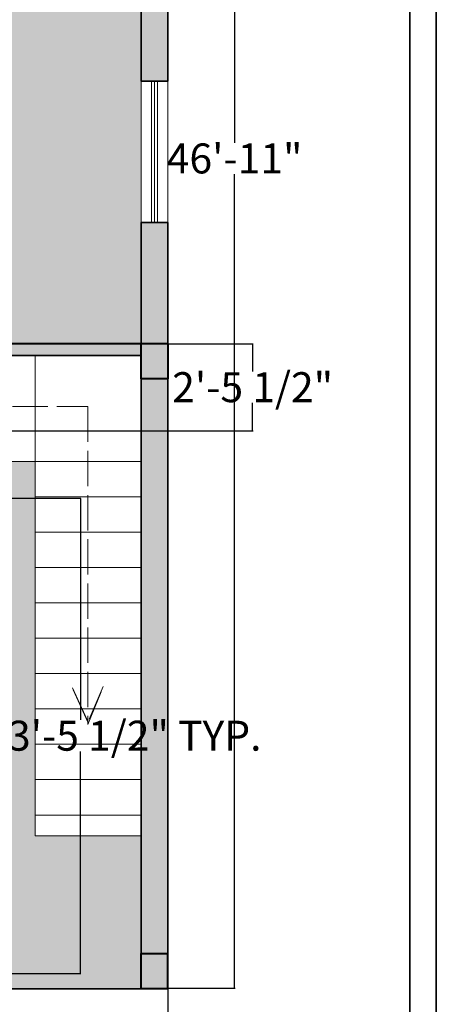
# Model space of a CAD drawing. Units: inches. Extents: x 1077 to 2505, y 1892 to 2728.
# Tile 24 of 26: x 2364 to 2505, y 2089 to 2423. Entities that reach past the tile are written whole.
import ezdxf

# ---------------------------------------------------------------- set-up
doc = ezdxf.new("R2010")
doc.units = ezdxf.units.IN
doc.linetypes.add('ACAD_ISO02W100', pattern=[15, 12, -3])
doc.layers.get('Defpoints').update_dxf_attribs({"color": 220, "linetype": 'ACAD_ISO02W100'})
for name, color, linetype, lineweight in [('A-ANNO-DIMS', 2, 'Continuous', 18), ('A-ANNO-STRS', 220, 'ACAD_ISO02W100', 13), ('A-ANNO-TTLB', 7, 'Continuous', 35), ('A-COLS', 7, 'Continuous', 40), ('A-FLOR-STRS', 7, 'Continuous', 18), ('A-WALL-PATT', 7, 'Continuous', 9), ('WALL', 7, 'Continuous', 35), ('WINDOW', 160, 'Continuous', 13)]:
    doc.layers.add(name, color=color, linetype=linetype, lineweight=lineweight)
doc.layers.add('A-FLOR-PATT', color=254, linetype='Continuous', lineweight=9, true_color=0xd7ebd2)
doc.styles.get("Standard").update_dxf_attribs({"font": 'arial.ttf'})
doc.dimstyles.get("Standard").update_dxf_attribs({"dimtxt": 10.18, "dimasz": 0.18, "dimexe": 0.18, "dimexo": 0.0625, "dimgap": 0.09, "dimtad": 0, "dimtih": 1, "dimtoh": 1, "dimdec": 0, "dimzin": 0, "dimdsep": 46, "dimlunit": 3, "dimtxsty": 'Standard', "dimcen": 0.09, "dimadec": 0, "dimazin": 0, "dimtfac": 1, "dimtdec": 0, "dimtofl": 0, "dimtmove": 0, "dimatfit": 3, "dimfxl": 1, "dimtolj": 1, "dimtzin": 0, "dimarcsym": 0})

# ---------------------------------------------------------------- blocks, each defined once
blk = doc.blocks.new('C1')
h = blk.add_hatch(color=256)
h.dxf.hatch_style = 1
h.paths.add_polyline_path([(1668.56, 2445.41), (1677.56, 2445.41), (1677.56, 2457.41), (1668.56, 2457.41)])
for p, q in [((1668.56, 2457.41), (1677.56, 2457.41)), ((1668.56, 2445.41), (1668.56, 2457.41)), ((1677.56, 2457.41), (1677.56, 2445.41)), ((1677.56, 2445.41), (1668.56, 2445.41))]:
    blk.add_line(p, q)
blk = doc.blocks.new('*D19')
at = {"layer": 'A-ANNO-DIMS', "color": 0, "lineweight": -2, "transparency": 16777216}
for p, q in [((2412.91, 2657.64), (2436.75, 2657.64)), ((2436.57, 2657.46), (2436.57, 2381.28)), ((2436.57, 2094.52), (2436.57, 2370.7)), ((2412.91, 2094.34), (2436.75, 2094.34))]:
    blk.add_line(p, q, dxfattribs=at)
at = {"layer": 'A-ANNO-DIMS', "color": 0, "transparency": 16777216}
for points in [[(2436.54, 2657.46), (2436.6, 2657.46), (2436.57, 2657.64)], [(2436.54, 2094.52), (2436.6, 2094.52), (2436.57, 2094.34)]]:
    blk.add_solid(points, dxfattribs=at)
at = {"layer": 'Defpoints', "color": 0, "transparency": 16777216}
for p in [(2412.85, 2657.64), (2412.85, 2094.34), (2436.57, 2094.34)]:
    blk.add_point(p, dxfattribs=at)
at = {"layer": 'A-ANNO-DIMS', "color": 0, "transparency": 16777216, "insert": (2436.57, 2375.99), "char_height": 10.18, "attachment_point": 5}
blk.add_mtext('\\A1;46\'-11"', dxfattribs=at)
blk = doc.blocks.new('WINDOW-48-EXT')
for p, q in [((0, 48), (0, 0)), ((3.5, 48), (3.5, 0)), ((4.5, 48), (4.5, 0)), ((5.5, 48), (5.5, 0)), ((9, 0), (9, 48))]:
    blk.add_line(p, q)
blk = doc.blocks.new('STAIR-PLAN-RETURN')
for p, q in [((0, 163.08), (0, 127.08)), ((12, 163.08), (12, 127.08)), ((24, 163.08), (24, 127.08)), ((36, 163.08), (36, 0)), ((36, 163.08), (36, 127.08)), ((0, 127.08), (72, 127.08)), ((36, 115.08), (72, 115.08)), ((36, 103.08), (72, 103.08)), ((36, 91.08), (72, 91.08)), ((36, 79.08), (72, 79.08)), ((36, 67.08), (72, 67.08)), ((36, 55.08), (72, 55.08)), ((36, 43.08), (72, 43.08)), ((36, 31.08), (72, 31.08)), ((36, 19.08), (72, 19.08)), ((36, 7.08), (72, 7.08)), ((72, 0), (36, 0))]:
    blk.add_line(p, q)
blk = doc.blocks.new('STAIR-DIRECTION')
for p, q in [((0, 107.9), (70.51, 107.9)), ((70.51, 107.9), (70.51, 0)), ((70.51, 0.8), (65.28, 12.48)), ((65.28, 12.48), (70.51, 1.21)), ((70.51, 0), (75.75, 12.88)), ((75.75, 12.88), (70.51, 0.8))]:
    blk.add_line(p, q)
blk = doc.blocks.new('SHEET-FRAME-RESIDENTIAL')
for points in [[(0, 830.04), (543.52, 830.04), (543.52, 0), (0, 0)], [(9, 821.04), (534.52, 821.04), (534.52, 9), (9, 9)]]:
    blk.add_lwpolyline(points, close=True)
blk = doc.blocks.new('*D56')
at = {"layer": 'A-ANNO-DIMS', "color": 0, "lineweight": -2, "transparency": 16777216}
for p, q in [((2360.05, 2260.72), (2384.37, 2260.72)), ((2384.19, 2260.54), (2384.19, 2185.41)), ((2384.19, 2099.57), (2384.19, 2174.7)), ((2360.05, 2099.39), (2384.37, 2099.39))]:
    blk.add_line(p, q, dxfattribs=at)
at = {"layer": 'A-ANNO-DIMS', "color": 0, "transparency": 16777216}
for points in [[(2384.16, 2260.54), (2384.22, 2260.54), (2384.19, 2260.72)], [(2384.16, 2099.57), (2384.22, 2099.57), (2384.19, 2099.39)]]:
    blk.add_solid(points, dxfattribs=at)
at = {"layer": 'Defpoints', "color": 0, "transparency": 16777216}
for p in [(2359.99, 2260.72), (2384.19, 2260.72), (2359.99, 2099.39)]:
    blk.add_point(p, dxfattribs=at)
at = {"layer": 'A-ANNO-DIMS', "color": 0, "transparency": 16777216, "insert": (2384.19, 2180.06), "char_height": 10.18, "attachment_point": 5}
blk.add_mtext('\\A1;CAR 13\'-5 1/2" TYP.', dxfattribs=at)
blk = doc.blocks.new('*D57')
at = {"layer": 'A-ANNO-DIMS', "color": 0, "lineweight": -2, "transparency": 16777216}
for p, q in [((2293.39, 2099.33), (2293.39, 2075.01)), ((2359.99, 2099.33), (2359.99, 2075.01)), ((2293.57, 2075.19), (2359.81, 2075.19)), ((2359.99, 2075.19), (2360.17, 2075.19))]:
    blk.add_line(p, q, dxfattribs=at)
at = {"layer": 'A-ANNO-DIMS', "color": 0, "transparency": 16777216}
for points in [[(2293.57, 2075.22), (2293.57, 2075.16), (2293.39, 2075.19)], [(2359.81, 2075.22), (2359.81, 2075.16), (2359.99, 2075.19)]]:
    blk.add_solid(points, dxfattribs=at)
at = {"layer": 'Defpoints', "color": 0, "transparency": 16777216}
for p in [(2293.39, 2099.39), (2359.99, 2099.39), (2359.99, 2075.19)]:
    blk.add_point(p, dxfattribs=at)
at = {"layer": 'A-ANNO-DIMS', "color": 0, "transparency": 16777216, "insert": (2403.15, 2075.19), "char_height": 10.18, "attachment_point": 5}
blk.add_mtext('\\A1;5\'-6 1/2" TYP.', dxfattribs=at)
blk = doc.blocks.new('*D63')
at = {"layer": 'A-ANNO-DIMS', "color": 0, "lineweight": -2, "transparency": 16777216}
for p, q in [((2035.85, 2094.07), (2035.85, 2065.11)), ((2413.85, 2094.07), (2413.85, 2065.11)), ((2036.03, 2065.29), (2207.27, 2065.29)), ((2413.67, 2065.29), (2242.42, 2065.29))]:
    blk.add_line(p, q, dxfattribs=at)
at = {"layer": 'A-ANNO-DIMS', "color": 0, "transparency": 16777216}
for points in [[(2036.03, 2065.32), (2036.03, 2065.26), (2035.85, 2065.29)], [(2413.67, 2065.32), (2413.67, 2065.26), (2413.85, 2065.29)]]:
    blk.add_solid(points, dxfattribs=at)
at = {"layer": 'Defpoints', "color": 0, "transparency": 16777216}
for p in [(2035.85, 2094.14), (2413.85, 2094.14), (2413.85, 2065.29)]:
    blk.add_point(p, dxfattribs=at)
at = {"layer": 'A-ANNO-DIMS', "color": 0, "transparency": 16777216, "insert": (2224.85, 2065.29), "char_height": 10.18, "attachment_point": 5}
blk.add_mtext('\\A1;31\'-6"', dxfattribs=at)
blk = doc.blocks.new('*D72')
at = {"layer": 'A-ANNO-DIMS', "color": 0, "lineweight": -2, "transparency": 16777216}
for p, q in [((2280.86, 2313.12), (2442.88, 2313.12)), ((2442.7, 2312.94), (2442.7, 2303.7)), ((2442.7, 2283.76), (2442.7, 2292.99)), ((2285.24, 2283.58), (2442.88, 2283.58))]:
    blk.add_line(p, q, dxfattribs=at)
at = {"layer": 'A-ANNO-DIMS', "color": 0, "transparency": 16777216}
for points in [[(2442.67, 2312.94), (2442.73, 2312.94), (2442.7, 2313.12)], [(2442.67, 2283.76), (2442.73, 2283.76), (2442.7, 2283.58)]]:
    blk.add_solid(points, dxfattribs=at)
at = {"layer": 'Defpoints', "color": 0, "transparency": 16777216}
for p in [(2280.8, 2313.12), (2285.18, 2283.58), (2442.7, 2283.58)]:
    blk.add_point(p, dxfattribs=at)
at = {"layer": 'A-ANNO-DIMS', "color": 0, "transparency": 16777216, "insert": (2442.7, 2298.35), "char_height": 10.18, "attachment_point": 5}
blk.add_mtext('\\A1;2\'-5 1/2"', dxfattribs=at)

msp = doc.modelspace()

# ---------------------------------------------------------------- hatches: boundary and pattern name
at = {"layer": 'A-FLOR-PATT', "transparency": 33554559}
h = msp.add_hatch(color=256, dxfattribs=at)
h.dxf.hatch_style = 1
h.paths.add_polyline_path([(2252.85, 2583.14), (2232.15, 2583.14), (2208.15, 2583.17), (2208.15, 2583.14), (2186.85, 2583.14), (2186.85, 2486.14), (2186.85, 2475.14), (2182.85, 2475.14), (2182.85, 2521.11), (2164.84, 2521.11), (2164.84, 2583.14), (2126.63, 2583.14), (2078.63, 2583.13), (2078.63, 2583.14), (2044.85, 2583.14), (2044.85, 2439.14), (2146.85, 2439.14), (2146.85, 2435.14), (2120.85, 2435.14), (2044.85, 2435.14), (2044.85, 2401), (2044.85, 2401), (2044.85, 2377), (2044.85, 2377), (2044.85, 2313.14), (2116.85, 2313.14), (2116.85, 2405.14), (2120.85, 2405.14), (2120.85, 2313.14), (2146.85, 2313.14), (2146.85, 2312.21), (2182.85, 2312.21), (2182.85, 2313.14), (2186.85, 2313.14), (2186.85, 2312.21), (2222.85, 2312.21), (2222.85, 2313.14), (2289.85, 2313.14), (2289.85, 2094.14), (2404.85, 2094.14), (2404.85, 2146.06), (2368.85, 2146.06), (2368.85, 2273.14), (2332.85, 2273.14), (2332.85, 2309.14), (2325.85, 2309.14), (2325.85, 2313.14), (2404.85, 2313.14), (2404.85, 2354.2), (2404.85, 2402.2), (2404.85, 2435.14), (2292.85, 2435.14), (2292.85, 2439.14), (2333.66, 2439.14), (2333.66, 2457.16), (2404.85, 2457.16), (2404.85, 2583.14), (2356.85, 2583.14), (2356.85, 2592.14), (2404.85, 2592.14), (2404.85, 2648.14), (2375.5, 2648.14), (2375.5, 2648.03), (2351.47, 2648.03), (2351.47, 2648.14), (2326.85, 2648.14), (2326.85, 2583.14), (2256.85, 2583.14), (2256.85, 2435.14), (2182.85, 2435.14), (2182.85, 2439.14), (2186.85, 2439.14), (2252.85, 2439.14), (2252.85, 2486.14), (2216.85, 2486.14), (2216.85, 2490.14), (2252.85, 2490.14)])
h.paths.add_polyline_path([(2214.97, 2488.05), (2212.97, 2488.05), (2212.97, 2487.05, 0.414214), (2213.97, 2486.05), (2201.97, 2486.05), (2201.97, 2483.04), (2200.58, 2483.04), (2200.58, 2486.05), (2187.97, 2486.05, -0.414214), (2186.97, 2487.05), (2186.97, 2490.05), (2188.97, 2490.05), (2188.97, 2516.05, -0.446908)], flags=16)
h.paths.add_polyline_path([(2162.4, 2565.16), (2146.2, 2565.16), (2146.2, 2581.36), (2162.4, 2581.36)], flags=16)
h.paths.add_polyline_path([(2161.5, 2566.06), (2147.1, 2566.06), (2147.1, 2580.46), (2161.5, 2580.46)], flags=0)
h.paths.add_polyline_path([(2145.3, 2506.66, -0.414214), (2144.4, 2505.76), (2122.45, 2505.76), (2081.4, 2505.76, -0.414214), (2080.5, 2506.66), (2080.5, 2563.14), (2080.5, 2577.72), (2080.5, 2581.36), (2145.3, 2581.36), (2145.3, 2577.72), (2144.4, 2577.72, -0.414214), (2145.3, 2576.82)], flags=16)
h.paths.add_polyline_path([(2150.3, 2575.03, -1), (2158.24, 2575.03, -1)], flags=0)
h.paths.add_polyline_path([(2150.64, 2575.03, -1), (2157.89, 2575.03, -1)], flags=0)
h.paths.add_polyline_path([(2180.11, 2468.19), (2180.11, 2437.69), (2180.36, 2436.69), (2180.36, 2437.69), (2179.11, 2437.69), (2179.11, 2468.17, 0.404641), (2149.61, 2437.69), (2149.36, 2436.69, -0.414214), (2148.86, 2436.19), (2148.36, 2436.19), (2148.36, 2435.69, -0.414214), (2147.86, 2435.19), (2146.86, 2435.19), (2146.86, 2440.19), (2147.86, 2440.19, -0.414214), (2148.36, 2439.69), (2148.36, 2439.19), (2148.86, 2439.19, -0.414214), (2149.36, 2438.69), (2149.61, 2437.69, -0.414214)], flags=16)
h.paths.add_polyline_path([(2145.14, 2554.26, 0.292232), (2136.49, 2542.78, 0.052719), (2081.25, 2554.26), (2080.6, 2554.26), (2080.6, 2563.14), (2081.25, 2563.14), (2102.73, 2563.14, -0.117785), (2103.09, 2563.91, -0.059418), (2112.19, 2573, -0.379859), (2114.6, 2572.86, -0.02509), (2118.73, 2569.3, -0.025935), (2122.97, 2573, -0.379859), (2125.38, 2572.86, -0.061767), (2134.84, 2563.41, -0.069393), (2135.14, 2563.14), (2145.14, 2563.14)], flags=0)
h.paths.add_polyline_path([(2120.79, 2554.26), (2117.88, 2554.26, -0.015371), (2115.33, 2552.11, -0.429576), (2112.69, 2552.04, -0.016036), (2110.01, 2554.26), (2080.6, 2554.26), (2080.6, 2560.4), (2104.1, 2560.4, 0.055344), (2112.69, 2552.04, 0.331768), (2114.84, 2551.72, 0.027343), (2119.32, 2555.62, 0.00919)], flags=0)
h.paths.add_polyline_path([(2152.88, 2574.32), (2154.19, 2575.07), (2154.19, 2576.58, 0.399698), (2152.71, 2575.03, 0.119004)], flags=0)
h.paths.add_polyline_path([(2152.53, 2575.03, -1), (2156, 2575.03, -1)], flags=0)
h.paths.add_polyline_path([(2154.27, 2574.94), (2154.34, 2574.98), (2154.34, 2575.07), (2154.3, 2575.09), (2154.23, 2574.96)], flags=0)
h.paths.add_polyline_path([(2259.6, 2468.17, -0.414214), (2290.1, 2437.67), (2290.35, 2438.67), (2290.1, 2437.67, 0.404641), (2260.6, 2468.15), (2260.6, 2437.67), (2259.35, 2437.67), (2259.35, 2436.67, -0.414214), (2258.85, 2436.17), (2258.35, 2436.17), (2258.35, 2435.67, -0.414214), (2257.85, 2435.17), (2256.85, 2435.17), (2256.85, 2440.17), (2257.85, 2440.17, -0.414214), (2258.35, 2439.67), (2258.35, 2439.17), (2258.85, 2439.17, -0.414214), (2259.35, 2438.67)], flags=16)
h.paths.add_polyline_path([(2327.48, 2541.19, -0.414214), (2328.38, 2542.09), (2384.85, 2542.09), (2399.43, 2542.09), (2403.08, 2542.09), (2403.08, 2477.29), (2399.43, 2477.29), (2399.43, 2478.19, -0.414214), (2398.53, 2477.29), (2328.38, 2477.29, -0.414214), (2327.48, 2478.19), (2327.48, 2500.14)], flags=16)
h.paths.add_polyline_path([(2340.38, 2542.09, 0.253465), (2337.43, 2532.13, 0.2538), (2327.47, 2529.17)], flags=16)
h.paths.add_polyline_path([(2080.5, 2518.67, 0.253465), (2090.46, 2515.72, 0.2538), (2093.42, 2505.75)], flags=16)
h.paths.add_polyline_path([(2327.09, 2584.7), (2327.09, 2587.7), (2329.09, 2587.7), (2329.09, 2613.7, -0.01951), (2331.09, 2613.66), (2331.09, 2585.7), (2331.09, 2584.7, -0.414214), (2330.09, 2583.7), (2328.09, 2583.7, -0.414214)], flags=16)
h.paths.add_polyline_path([(2239.78, 2404.11), (2252.36, 2404.11), (2252.36, 2405.72), (2239.78, 2405.72)], flags=16)
h.paths.add_polyline_path([(2237.26, 2403.16), (2237.26, 2395.8), (2237.82, 2395.8), (2237.82, 2402.03, -0.41429), (2238.38, 2402.59), (2253.79, 2402.59, -0.414213), (2254.35, 2402.03), (2254.35, 2395.8), (2254.91, 2395.8), (2254.91, 2403.16)], flags=16)
h.paths.add_polyline_path([(2120.69, 2434.12), (2120.69, 2432.12, -0.414214), (2119.69, 2431.12), (2118.69, 2431.12), (2090.73, 2431.12, 0.400854), (2116.69, 2407.02), (2116.69, 2407.12), (2118.69, 2407.12, -0.446908), (2090.69, 2433.12), (2116.69, 2433.12), (2116.69, 2435.12), (2119.69, 2435.12, -0.414214)], flags=16)
h.paths.add_polyline_path([(2262.11, 2404.11), (2274.69, 2404.11), (2274.69, 2405.72), (2262.11, 2405.72)], flags=16)
h.paths.add_polyline_path([(2259.59, 2403.16), (2262.11, 2404.11), (2274.69, 2404.11), (2277.24, 2403.16)], flags=16)
h.paths.add_polyline_path([(2289.58, 2389.14), (2289.58, 2376.57), (2291.19, 2376.57), (2291.19, 2389.14)], flags=16)
h.paths.add_polyline_path([(2288.62, 2391.67), (2281.15, 2391.67), (2281.15, 2391.11), (2287.5, 2391.11, -0.41429), (2288.06, 2390.54), (2288.06, 2375.14, -0.414237), (2287.5, 2374.58), (2281.15, 2374.58), (2281.15, 2374.01), (2288.62, 2374.01)], flags=16)
h.paths.add_polyline_path([(2274.69, 2357.14), (2274.69, 2355.52), (2276.22, 2355.52, 0.414236), (2277.24, 2356.54), (2277.24, 2358.09)], flags=16)
h.paths.add_polyline_path([(2252.36, 2357.14), (2252.36, 2355.52), (2253.89, 2355.52, 0.414235), (2254.91, 2356.54), (2254.91, 2358.09)], flags=16)
h.paths.add_polyline_path([(2224.02, 2376.03), (2222.41, 2376.03), (2222.41, 2374.5, 0.414235), (2223.43, 2373.48), (2224.98, 2373.48)], flags=16)
h.paths.add_polyline_path([(2276.68, 2365.45), (2276.68, 2359.22, -0.41419), (2276.12, 2358.66), (2260.71, 2358.66, -0.414137), (2260.15, 2359.22), (2260.15, 2365.45), (2254.35, 2365.45), (2254.35, 2359.22, -0.414189), (2253.79, 2358.66), (2238.38, 2358.66, -0.414137), (2237.82, 2359.22), (2237.82, 2365.45)], flags=16)
h.paths.add_polyline_path([(2079.6, 2565.16), (2063.4, 2565.16), (2063.4, 2581.36), (2079.6, 2581.36)], flags=16)
h.paths.add_polyline_path([(2078.7, 2566.06), (2064.3, 2566.06), (2064.3, 2580.46), (2078.7, 2580.46)], flags=0)
h.paths.add_polyline_path([(2339.31, 2583.7), (2339.31, 2586.71), (2340.7, 2586.71), (2340.7, 2583.7), (2342.09, 2583.7), (2342.09, 2580.7), (2340.7, 2580.7), (2340.7, 2583.7)], flags=16)
h.paths.add_polyline_path([(2123.69, 2421.51), (2123.69, 2420.12), (2120.69, 2420.12), (2120.69, 2421.51), (2117.68, 2421.51), (2117.68, 2422.89), (2120.69, 2422.89), (2120.69, 2421.51)], flags=16)
h.paths.add_polyline_path([(2067.57, 2575.03, -1), (2075.51, 2575.03, -1)], flags=0)
h.paths.add_polyline_path([(2067.92, 2575.03, -1), (2075.17, 2575.03, -1)], flags=0)
h.paths.add_polyline_path([(2070.16, 2574.32), (2071.47, 2575.07), (2071.47, 2576.58, 0.399698), (2069.99, 2575.03, 0.119004)], flags=0)
h.paths.add_polyline_path([(2069.81, 2575.03, -1), (2073.28, 2575.03, -1)], flags=0)
h.paths.add_polyline_path([(2071.54, 2574.94), (2071.62, 2574.89), (2071.62, 2574.98)], flags=0)
h.paths.add_polyline_path([(2364.5, 2486.1, 0.052719), (2375.98, 2541.34), (2375.98, 2541.99), (2384.85, 2541.99), (2384.85, 2541.34), (2384.85, 2519.86, -0.117785), (2385.62, 2519.51, -0.059418), (2394.72, 2510.41, -0.379859), (2394.58, 2507.99, -0.02509), (2391.01, 2503.87, -0.025935), (2394.72, 2499.62, -0.379859), (2394.58, 2497.21, -0.061767), (2385.12, 2487.75, -0.069393), (2384.85, 2487.45), (2384.85, 2477.45), (2375.98, 2477.45, 0.292232)], flags=0)
h.paths.add_polyline_path([(2373.75, 2509.9, -0.016036), (2375.98, 2512.58), (2375.98, 2541.99), (2382.12, 2541.99), (2382.12, 2518.49, 0.055344), (2373.75, 2509.9, 0.331768), (2373.44, 2507.75, 0.027343), (2377.33, 2503.27, 0.00919), (2375.98, 2501.8), (2375.98, 2504.71, -0.015371), (2373.82, 2507.26, -0.429576)], flags=0)
h.paths.add_polyline_path([(2356.95, 2631.48, -0.171636), (2360.13, 2636.99), (2360.13, 2639.35), (2356, 2639.35, -0.414214), (2355.01, 2640.34), (2355.01, 2646.64, -0.414214), (2356, 2647.62), (2372.14, 2647.62, -0.414214), (2373.13, 2646.64), (2373.13, 2640.34, -0.414214), (2372.14, 2639.35), (2368.01, 2639.35), (2368.01, 2636.99, -0.171636), (2371.2, 2631.48, -0.258205), (2366.63, 2620.45), (2361.51, 2620.45, -0.258205)], flags=16)
h.paths.add_polyline_path([(2358.52, 2631.48, -0.171636), (2361.71, 2636.99), (2366.43, 2636.99, -0.171636), (2369.62, 2631.48, -0.210384), (2366.67, 2622), (2361.47, 2622, -0.210384)], flags=0)
h.paths.add_polyline_path([(2386.88, 2542.99), (2386.88, 2559.19), (2403.08, 2559.19), (2403.08, 2542.99)], flags=16)
h.paths.add_polyline_path([(2387.78, 2543.89), (2387.78, 2558.29), (2402.18, 2558.29), (2402.18, 2543.89)], flags=0)
h.paths.add_polyline_path([(2392.77, 2551.05, -1), (2400.71, 2551.05, -1)], flags=0)
h.paths.add_polyline_path([(2393.11, 2551.05, -1), (2400.37, 2551.05, -1)], flags=0)
h.paths.add_polyline_path([(2386.88, 2476.39), (2403.08, 2476.39), (2403.08, 2460.19), (2386.88, 2460.19)], flags=16)
h.paths.add_polyline_path([(2398.48, 2550.97), (2398.3, 2550.97, -0.544606), (2396.03, 2549.66), (2395.94, 2549.51, 0.547962)], flags=0)
h.paths.add_polyline_path([(2387.78, 2475.49), (2402.18, 2475.49), (2402.18, 2461.09), (2387.78, 2461.09)], flags=0)
h.paths.add_polyline_path([(2396.79, 2551.12), (2396.74, 2551.2), (2396.7, 2551.12)], flags=0)
h.paths.add_polyline_path([(2400.71, 2468.32, -1), (2392.77, 2468.32, -1)], flags=0)
h.paths.add_polyline_path([(2400.37, 2468.32, -1), (2393.11, 2468.32, -1)], flags=0)
h.paths.add_polyline_path([(2398.48, 2468.25), (2398.3, 2468.25, -0.544606), (2396.03, 2466.94), (2395.94, 2466.78, 0.547962)], flags=0)
h.paths.add_polyline_path([(2396.79, 2468.4), (2396.74, 2468.48), (2396.7, 2468.4)], flags=0)
h.paths.add_polyline_path([(2292.64, 2341.23, -0.414214), (2323.14, 2310.73), (2323.39, 2311.73), (2323.14, 2310.73, 0.404641), (2293.64, 2341.21), (2293.64, 2310.73), (2292.39, 2310.73), (2292.39, 2309.73, -0.414214), (2291.89, 2309.23), (2291.39, 2309.23), (2291.39, 2308.73, -0.414214), (2290.89, 2308.23), (2289.89, 2308.23), (2289.89, 2313.23), (2290.89, 2313.23, -0.414214), (2291.39, 2312.73), (2291.39, 2312.23), (2291.89, 2312.23, -0.414214), (2292.39, 2311.73)], flags=16)
h.paths.add_polyline_path([(2389.45, 2641.69), (2392.75, 2641.69), (2392.75, 2641.87), (2389.45, 2641.87)], flags=16)
edge = h.paths.add_edge_path(flags=16)
edge.add_arc((2393.3, 2638.65), 0.183, 270, 360)
edge.add_line((2393.49, 2638.65), (2393.49, 2645.8))
edge.add_line((2393.49, 2645.8), (2395.61, 2645.8))
edge.add_line((2395.61, 2645.8), (2395.61, 2647.8))
edge.add_line((2395.61, 2647.8), (2390.57, 2647.8))
edge.add_line((2390.57, 2647.8), (2390.57, 2645.8))
edge.add_line((2390.57, 2645.8), (2392.19, 2645.8))
edge.add_line((2392.19, 2645.8), (2392.19, 2644.98))
edge.add_line((2392.19, 2644.98), (2391.02, 2644.98))
edge.add_line((2391.02, 2644.98), (2391.02, 2645.8))
edge.add_line((2391.02, 2645.8), (2390.57, 2645.8))
edge.add_line((2390.57, 2645.8), (2390.57, 2647.8))
edge.add_line((2390.57, 2647.8), (2395.61, 2647.8))
edge.add_line((2395.61, 2647.8), (2395.61, 2647.32))
edge.add_line((2395.61, 2647.32), (2397.95, 2647.56))
edge.add_line((2397.95, 2647.56), (2397.95, 2647.8))
edge.add_line((2397.95, 2647.8), (2398.81, 2647.8))
edge.add_line((2398.81, 2647.8), (2398.81, 2647.23))
edge.add_line((2398.81, 2647.23), (2398.63, 2645.77))
edge.add_ellipse((2398.41, 2644.93), major_axis=(-1.08, 0), ratio=0.790849, start_angle=180, end_angle=255.2976, ccw=False)
edge.add_line((2399.49, 2644.93), (2399.49, 2644.36))
edge.add_ellipse((2398.41, 2644.36), major_axis=(-1.08, 0), ratio=0.790849, start_angle=0, end_angle=180, ccw=False)
edge.add_line((2397.32, 2644.36), (2397.33, 2644.85))
edge.add_ellipse((2398.41, 2644.93), major_axis=(-1.08, 0), ratio=0.790849, start_angle=284.7024, end_angle=364.0401, ccw=False)
edge.add_line((2398.1, 2645.73), (2398.1, 2647.23))
edge.add_line((2398.1, 2647.23), (2397.95, 2647.23))
edge.add_line((2397.95, 2647.23), (2395.61, 2646.99))
edge.add_line((2395.61, 2646.99), (2395.61, 2645.8))
edge.add_line((2395.61, 2645.8), (2393.49, 2645.8))
edge.add_line((2393.49, 2645.8), (2393.49, 2638.46))
edge.add_line((2393.49, 2638.46), (2393.3, 2638.46))
h.paths.add_polyline_path([(2353.64, 2256.32, -0.292371), (2356.22, 2253.81, -0.085148), (2358.52, 2214.83, -0.01331), (2357.59, 2104.48, -0.379287), (2354.54, 2101.26, -0.0502), (2298.86, 2101.26, -0.379287), (2295.81, 2104.48, -0.01331), (2294.88, 2214.83, -0.086132), (2297.28, 2254.24, -0.295116), (2299.9, 2256.76, -0.114238)], flags=16)
h.paths.add_polyline_path([(2352.48, 2211.82, -0.355389), (2354.02, 2208.08), (2350.26, 2195.63, -0.398275), (2346.44, 2193.45, 0.113332), (2306.96, 2193.45, -0.398275), (2303.14, 2195.63), (2299.38, 2208.08, -0.355394), (2300.92, 2211.82, -0.265725)], flags=0)
h.paths.add_polyline_path([(2297.68, 2201.7), (2303.26, 2187.65), (2303.26, 2166.61), (2298.16, 2163.24)], flags=0)
h.paths.add_polyline_path([(2355.78, 2201.7), (2355.31, 2163.24), (2350.2, 2166.61), (2350.2, 2187.65)], flags=0)
h.paths.add_polyline_path([(2303.26, 2164.35), (2303.26, 2143.1), (2298.44, 2128.54), (2298.19, 2161.01)], flags=0)
h.paths.add_polyline_path([(2350.2, 2164.35), (2355.28, 2161.01), (2355.03, 2128.54), (2350.2, 2143.1)], flags=0)
h.paths.add_polyline_path([(2347.2, 2136.38), (2351.71, 2113.65, -0.090102), (2301.76, 2113.63), (2306.27, 2136.37, 0.036636)], flags=0)
h.paths.add_polyline_path([(2304.86, 2165.32), (2354.76, 2165.32), (2354.76, 2183.87), (2304.86, 2183.87)], flags=8)
h.paths.add_polyline_path([(2053.76, 2360.82), (2103.97, 2360.82), (2103.97, 2394.41), (2053.76, 2394.41)], flags=24)
h.paths.add_polyline_path([(2153.41, 2366.23), (2211.12, 2366.23), (2211.12, 2399.82), (2153.41, 2399.82)], flags=24)
h.paths.add_polyline_path([(2258.04, 2477.83), (2327.95, 2477.83), (2327.95, 2511.42), (2258.04, 2511.42)], flags=24)
h.paths.add_polyline_path([(2182.1, 2454.46), (2252.27, 2454.46), (2252.27, 2473), (2182.1, 2473)], flags=24)
h.paths.add_polyline_path([(2192.4, 2537.41), (2246.99, 2537.41), (2246.99, 2571), (2192.4, 2571)], flags=24)
h.paths.add_polyline_path([(2083.07, 2465.98), (2152.99, 2465.98), (2152.99, 2499.56), (2083.07, 2499.56)], flags=24)
at = {"layer": 'A-WALL-PATT', "transparency": 33554585}
h = msp.add_hatch(color=256, dxfattribs=at)
h.dxf.hatch_style = 1
h.paths.add_polyline_path([(2044.85, 2429.98), (2035.85, 2429.98), (2035.85, 2401), (2044.85, 2401)])
h.paths.add_polyline_path([(2044.85, 2377), (2035.85, 2377), (2035.85, 2317.47), (2044.85, 2317.47)])
h.paths.add_polyline_path([(2085.45, 2159.14), (2044.85, 2159.14), (2044.85, 2225.64), (2035.85, 2225.64), (2035.85, 2106.16), (2044.85, 2106.16), (2044.85, 2150.14), (2085.45, 2150.14)])
h.paths.add_polyline_path([(2289.85, 2103.14), (2044.85, 2103.14), (2044.85, 2106.16), (2035.85, 2106.16), (2035.85, 2094.14), (2289.85, 2094.14)])
h.paths.add_polyline_path([(2413.85, 2354.2), (2404.85, 2354.2), (2404.85, 2354.2), (2404.85, 2313.14), (2325.85, 2313.14), (2325.85, 2309.14), (2404.85, 2309.14), (2404.85, 2094.14), (2413.85, 2094.14)])
h.paths.add_polyline_path([(2413.85, 2431.09), (2404.85, 2431.09), (2404.85, 2402.2), (2413.85, 2402.2)])
h.paths.add_polyline_path([(2404.85, 2439.14), (2292.85, 2439.14), (2292.85, 2435.14), (2404.85, 2435.14)])
h.paths.add_polyline_path([(2413.85, 2580.36), (2404.85, 2580.36), (2404.85, 2457.16), (2404.87, 2457.16), (2404.87, 2443.09), (2413.85, 2443.09)])
h.paths.add_polyline_path([(2413.85, 2645.09), (2404.85, 2645.09), (2404.85, 2592.36), (2413.85, 2592.36)])
h.paths.add_polyline_path([(2413.85, 2645.09), (2404.85, 2645.09), (2404.85, 2648.14), (2375.5, 2648.14), (2375.5, 2648.03), (2351.5, 2648.03), (2351.5, 2657.03), (2375.47, 2657.03), (2375.47, 2657.14), (2413.85, 2657.14)])
h.paths.add_polyline_path([(2351.47, 2657.14), (2326.92, 2657.14), (2326.92, 2648.14), (2351.47, 2648.14)])
h.paths.add_polyline_path([(2078.63, 2583.14), (2044.92, 2583.14), (2044.92, 2580.01), (2035.92, 2580.01), (2035.92, 2592.14), (2078.63, 2592.14)])
h.paths.add_polyline_path([(2180.39, 2592.14), (2126.63, 2592.14), (2126.63, 2583.14), (2180.39, 2583.14)])
h.paths.add_polyline_path([(2232.16, 2592.17), (2232.16, 2583.17), (2208.16, 2583.17), (2208.15, 2583.17), (2208.15, 2583.14), (2189.39, 2583.14), (2189.39, 2579.98), (2180.39, 2579.98), (2180.39, 2592.14), (2208.15, 2592.14), (2208.16, 2592.14), (2208.16, 2592.17)])
h.paths.add_polyline_path([(2250.27, 2592.14), (2232.16, 2592.14), (2232.16, 2583.14), (2250.27, 2583.14)], flags=17)
h.paths.add_polyline_path([(2326.85, 2648.14), (2326.92, 2657.14), (2317.85, 2657.14), (2317.85, 2592.14), (2250.27, 2592.14), (2250.27, 2583.14), (2252.85, 2583.14), (2252.85, 2490.14), (2216.85, 2490.14), (2216.85, 2486.14), (2252.85, 2486.14), (2252.85, 2439.14), (2186.85, 2439.14), (2182.85, 2439.14), (2182.85, 2435.14), (2256.85, 2435.14), (2256.85, 2583.14), (2326.85, 2583.14)])
h.paths.add_polyline_path([(2044.85, 2580.01), (2035.85, 2580.01), (2035.85, 2441.98), (2044.85, 2441.98)])

# ---------------------------------------------------------------- linework, layer by layer
at = {"layer": 'WALL'}
for p, q in [((2413.85, 2657.14), (2413.85, 2402.2)), ((2404.85, 2435.14), (2404.85, 2402.2)), ((2404.85, 2402.2), (2413.85, 2402.2)), ((2404.85, 2354.2), (2404.85, 2313.14)), ((2404.85, 2354.2), (2413.85, 2354.2)), ((2413.85, 2354.2), (2413.85, 2094.14)), ((2325.85, 2313.14), (2404.85, 2313.14)), ((2325.85, 2309.14), (2404.85, 2309.14)), ((2404.85, 2309.14), (2404.85, 2094.14)), ((2413.85, 2094.14), (2035.85, 2094.14))]:
    msp.add_line(p, q, dxfattribs=at)

# ---------------------------------------------------------------- block references
at = {"layer": 'A-ANNO-STRS'}
msp.add_blockref('STAIR-DIRECTION', (2316.18, 2183.85), dxfattribs=at)
at = {"layer": 'A-ANNO-TTLB'}
msp.add_blockref('SHEET-FRAME-RESIDENTIAL', (1961.57, 1898.25), dxfattribs=at)
at = {"layer": 'A-COLS'}
for p in [(736.29, -144.23), (736.28, -351.24)]:
    msp.add_blockref('C1', p, dxfattribs=at)
at = {"layer": 'A-FLOR-STRS'}
msp.add_blockref('STAIR-PLAN-RETURN', (2332.85, 2146.06), dxfattribs=at)
at = {"layer": 'WINDOW', "rotation": 180}
msp.add_blockref('WINDOW-48-EXT', (2413.85, 2402.2), dxfattribs=at)

# ---------------------------------------------------------------- dimensions: what is measured, and where the dimension line sits
at = {"layer": 'A-ANNO-DIMS'}
for base, p1, p2, override, picture, middle in [((2436.57, 2094.34), (2412.85, 2657.64), (2412.85, 2094.34), {"dimclrd": 0, "dimclre": 0, "dimclrt": 0}, '*D19', (2436.57, 2375.99)), ((2442.7, 2283.58), (2280.8, 2313.12), (2285.18, 2283.58), {"dimdec": 1, "dimlfac": 1, "dimrnd": 0, "dimzin": 1, "dimdsep": 46, "dimlunit": 4, "dimfrac": 2}, '*D72', (2442.7, 2298.35))]:
    dim = msp.add_linear_dim(base=base, p1=p1, p2=p2, angle=90, dimstyle='Standard', override=override, dxfattribs=at)
    dim.commit()
    dim.dimension.update_dxf_attribs({"geometry": picture, "text_midpoint": middle})
dim = msp.add_linear_dim(base=(2384.19, 2260.72), p1=(2359.99, 2099.39), p2=(2359.99, 2260.72), angle=90, text='CAR <> TYP.', dimstyle='Standard', override={"dimdec": 1, "dimlfac": 1, "dimrnd": 0, "dimzin": 1, "dimdsep": 46, "dimlunit": 4, "dimfrac": 2}, dxfattribs=at)
dim.commit()
dim.dimension.update_dxf_attribs({"geometry": '*D56', "text_midpoint": (2384.19, 2180.06)})
dim = msp.add_linear_dim(base=(2359.99, 2075.19), p1=(2293.39, 2099.39), p2=(2359.99, 2099.39), text='<> TYP.', dimstyle='Standard', override={"dimdec": 1, "dimlfac": 1, "dimrnd": 0, "dimzin": 1, "dimdsep": 46, "dimlunit": 4, "dimfrac": 2}, dxfattribs=at)
dim.commit()
dim.dimension.update_dxf_attribs({"geometry": '*D57', "text_midpoint": (2403.15, 2075.19)})
dim = msp.add_linear_dim(base=(2413.85, 2065.29), p1=(2035.85, 2094.14), p2=(2413.85, 2094.14), dimstyle='Standard', override={"dimdec": 1, "dimlfac": 1, "dimrnd": 0, "dimzin": 1, "dimdsep": 46, "dimlunit": 4, "dimfrac": 2}, dxfattribs=at)
dim.commit()
dim.dimension.update_dxf_attribs({"geometry": '*D63', "text_midpoint": (2224.85, 2065.29)})

doc.saveas('drawing.dxf')
